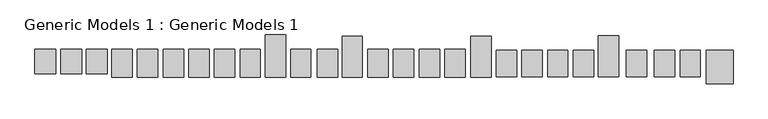
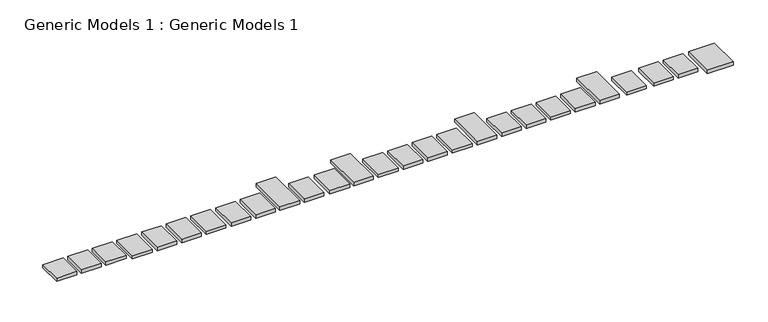
"""IFC4 building model written with IfcOpenShell, lengths in millimetres: proxy geometry, Generic Models 1 : Generic Models 1."""

from ifc_helpers import new_model, si_unit, origin, origin_with_axes, place, context, project, spatial, polyline, outline, extrude, source, transform, mapped, element, save


def generic_models_1_generic_models_1_84634830(model_context):
    return source(origin(), model_context, "Body", "SweptSolid", [
        extrude(outline(polyline([(-48968.7556936, 28500.6976136), (-48968.7556936, 27967.2976136), (-49425.9556936, 27967.2976136), (-49425.9556936, 28500.6976136), (-48968.7556936, 28500.6976136)])), origin_with_axes(), (0.0, 0.0, 1.0), 79.9703125),
        extrude(outline(polyline([(-48409.9556936, 28500.6976136), (-48409.9556936, 27967.2976136), (-48867.1556936, 27967.2976136), (-48867.1556936, 28500.6976136), (-48409.9556936, 28500.6976136)])), origin_with_axes(), (0.0, 0.0, 1.0), 79.9703125),
        extrude(outline(polyline([(-47851.1556936, 28500.6976136), (-47851.1556936, 27967.2976136), (-48308.3556936, 27967.2976136), (-48308.3556936, 28500.6976136), (-47851.1556936, 28500.6976136)])), origin_with_axes(), (0.0, 0.0, 1.0), 79.9703125),
        extrude(outline(polyline([(-47305.0556936, 28500.6976136), (-47305.0556936, 27891.0976136), (-47749.5556936, 27891.0976136), (-47749.5556936, 28500.6976136), (-47305.0556936, 28500.6976136)])), origin_with_axes(), (0.0, 0.0, 1.0), 79.9703125),
        extrude(outline(polyline([(-46746.2556936, 28500.6976136), (-46746.2556936, 27891.0976136), (-47190.7556936, 27891.0976136), (-47190.7556936, 28500.6976136), (-46746.2556936, 28500.6976136)])), origin_with_axes(), (0.0, 0.0, 1.0), 79.9703125),
        extrude(outline(polyline([(-46187.4556936, 28500.6976136), (-46187.4556936, 27891.0976136), (-46631.9556936, 27891.0976136), (-46631.9556936, 28500.6976136), (-46187.4556936, 28500.6976136)])), origin_with_axes(), (0.0, 0.0, 1.0), 79.9703125),
        extrude(outline(polyline([(-45628.6556936, 28500.6976136), (-45628.6556936, 27891.0976136), (-46073.1556936, 27891.0976136), (-46073.1556936, 28500.6976136), (-45628.6556936, 28500.6976136)])), origin_with_axes(), (0.0, 0.0, 1.0), 79.9703125),
        extrude(outline(polyline([(-45069.8556936, 28500.6976136), (-45069.8556936, 27891.0976136), (-45514.3556936, 27891.0976136), (-45514.3556936, 28500.6976136), (-45069.8556936, 28500.6976136)])), origin_with_axes(), (0.0, 0.0, 1.0), 79.9703125),
        extrude(outline(polyline([(-44511.0556936, 28500.6976136), (-44511.0556936, 27891.0976136), (-44955.5556936, 27891.0976136), (-44955.5556936, 28500.6976136), (-44511.0556936, 28500.6976136)])), origin_with_axes(), (0.0, 0.0, 1.0), 79.9703125),
        extrude(outline(polyline([(-43961.1295622, 28818.1976136), (-43961.1295622, 27891.0976136), (-44405.6295622, 27891.0976136), (-44405.6295622, 28818.1976136), (-43961.1295622, 28818.1976136)])), origin_with_axes(), (0.0, 0.0, 1.0), 79.9703125),
        extrude(outline(polyline([(-43411.2034308, 28500.6976136), (-43411.2034308, 27891.0976136), (-43855.7034308, 27891.0976136), (-43855.7034308, 28500.6976136), (-43411.2034308, 28500.6976136)])), origin_with_axes(), (0.0, 0.0, 1.0), 79.9703125),
        extrude(outline(polyline([(-42827.0034308, 28500.6976136), (-42827.0034308, 27891.0976136), (-43271.5034308, 27891.0976136), (-43271.5034308, 28500.6976136), (-42827.0034308, 28500.6976136)])), origin_with_axes(), (0.0, 0.0, 1.0), 79.9703125),
        extrude(outline(polyline([(-42288.7585782, 28786.8874783), (-42288.7585782, 27891.0976136), (-42733.2585782, 27891.0976136), (-42733.2585782, 28786.8874783), (-42288.7585782, 28786.8874783)])), origin_with_axes(), (0.0, 0.0, 1.0), 79.9703125),
        extrude(outline(polyline([(-41727.0793432, 28500.6976136), (-41727.0793432, 27891.0976136), (-42171.5793432, 27891.0976136), (-42171.5793432, 28500.6976136), (-41727.0793432, 28500.6976136)])), origin_with_axes(), (0.0, 0.0, 1.0), 79.9703125),
        extrude(outline(polyline([(-41168.2793432, 28500.6976136), (-41168.2793432, 27891.0976136), (-41612.7793432, 27891.0976136), (-41612.7793432, 28500.6976136), (-41168.2793432, 28500.6976136)])), origin_with_axes(), (0.0, 0.0, 1.0), 79.9703125),
        extrude(outline(polyline([(-40609.4793432, 28500.6976136), (-40609.4793432, 27891.0976136), (-41053.9793432, 27891.0976136), (-41053.9793432, 28500.6976136), (-40609.4793432, 28500.6976136)])), origin_with_axes(), (0.0, 0.0, 1.0), 79.9703125),
        extrude(outline(polyline([(-40050.6793432, 28500.6976136), (-40050.6793432, 27891.0976136), (-40495.1793432, 27891.0976136), (-40495.1793432, 28500.6976136), (-40050.6793432, 28500.6976136)])), origin_with_axes(), (0.0, 0.0, 1.0), 79.9703125),
        extrude(outline(polyline([(-39484.8902004, 28788.9815809), (-39484.8902004, 27891.0976136), (-39929.3902004, 27891.0976136), (-39929.3902004, 28788.9815809), (-39484.8902004, 28788.9815809)])), origin_with_axes(), (0.0, 0.0, 1.0), 79.9703125),
        extrude(outline(polyline([(-38929.5066863, 28481.1274721), (-38929.5066863, 27903.2774721), (-39374.0066863, 27903.2774721), (-39374.0066863, 28481.1274721), (-38929.5066863, 28481.1274721)])), origin_with_axes(), (0.0, 0.0, 1.0), 79.9703125),
        extrude(outline(polyline([(-38370.7066863, 28481.1274721), (-38370.7066863, 27903.2774721), (-38815.2066863, 27903.2774721), (-38815.2066863, 28481.1274721), (-38370.7066863, 28481.1274721)])), origin_with_axes(), (0.0, 0.0, 1.0), 79.9703125),
        extrude(outline(polyline([(-37811.9066863, 28481.1274721), (-37811.9066863, 27903.2774721), (-38256.4066863, 27903.2774721), (-38256.4066863, 28481.1274721), (-37811.9066863, 28481.1274721)])), origin_with_axes(), (0.0, 0.0, 1.0), 79.9703125),
        extrude(outline(polyline([(-37253.1066863, 28481.1274721), (-37253.1066863, 27903.2774721), (-37697.6066863, 27903.2774721), (-37697.6066863, 28481.1274721), (-37253.1066863, 28481.1274721)])), origin_with_axes(), (0.0, 0.0, 1.0), 79.9703125),
        extrude(outline(polyline([(-36703.1805549, 28798.6274721), (-36703.1805549, 27903.2774721), (-37147.6805549, 27903.2774721), (-37147.6805549, 28798.6274721), (-36703.1805549, 28798.6274721)])), origin_with_axes(), (0.0, 0.0, 1.0), 79.9703125),
        extrude(outline(polyline([(-36092.1282806, 28487.2807874), (-36092.1282806, 27903.2774721), (-36536.6282806, 27903.2774721), (-36536.6282806, 28487.2807874), (-36092.1282806, 28487.2807874)])), origin_with_axes(), (0.0, 0.0, 1.0), 79.9703125),
        extrude(outline(polyline([(-35482.5282806, 28487.2807874), (-35482.5282806, 27903.2774721), (-35927.0282806, 27903.2774721), (-35927.0282806, 28487.2807874), (-35482.5282806, 28487.2807874)])), origin_with_axes(), (0.0, 0.0, 1.0), 79.9703125),
        extrude(outline(polyline([(-34923.7282806, 28487.2807874), (-34923.7282806, 27903.2774721), (-35368.2282806, 27903.2774721), (-35368.2282806, 28487.2807874), (-34923.7282806, 28487.2807874)])), origin_with_axes(), (0.0, 0.0, 1.0), 79.9703125),
        extrude(outline(polyline([(-34212.5282806, 28487.2807874), (-34212.5282806, 27750.6807874), (-34796.7282806, 27750.6807874), (-34796.7282806, 28487.2807874), (-34212.5282806, 28487.2807874)])), origin_with_axes(), (0.0, 0.0, 1.0), 79.9703125),
    ])


if __name__ == "__main__":
    model = new_model("IFC4")
    model_context = context("Model", 3, world=origin())
    ifc_project = project(units=[si_unit("LENGTHUNIT", "METRE", prefix="MILLI")], contexts=[model_context])
    site = spatial("IfcSite", under=ifc_project)
    building = spatial("IfcBuilding", under=site)
    placement = place(None, origin())
    generic_models_1_generic_models_1_shape = generic_models_1_generic_models_1_84634830(model_context)
    element("IfcBuildingElementProxy", 1, Name="Generic Models 1 : Generic Models 1", ObjectType="Generic Models 1 : Generic Models 1", at=placement, inside=building, context=model_context, shape_type="MappedRepresentation", body=[
        mapped(generic_models_1_generic_models_1_shape, transform((0.0, 0.0, 0.0), x_axis=(1.0, 0.0, 0.0), y_axis=(0.0, 1.0, 0.0), z_axis=(0.0, 0.0, 1.0))),
    ])
    save(model, "model.ifc")
